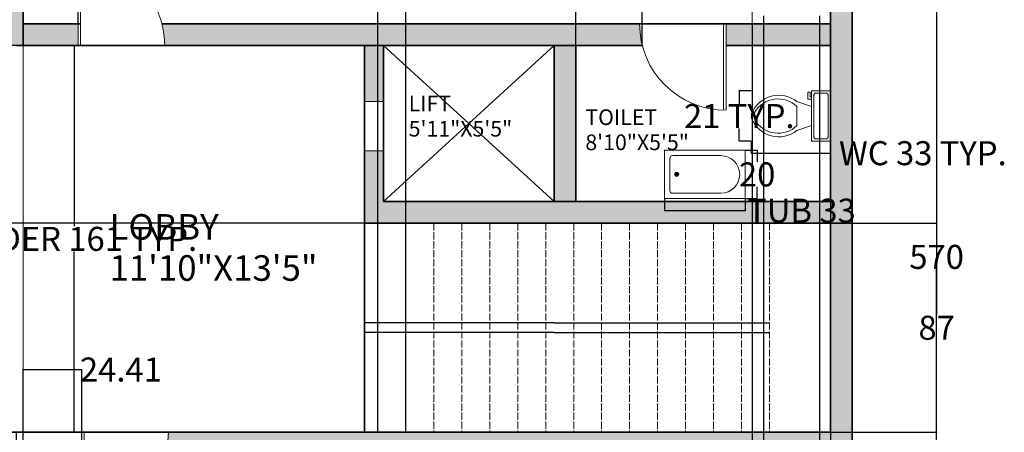
# Model space of a CAD drawing. Units: inches. Extents: x 409 to 1056, y 160 to 945.
# Tile 3 of 6: x 625 to 1035, y 453 to 624. Entities that reach past the tile are written whole.
import ezdxf

# ---------------------------------------------------------------- set-up
doc = ezdxf.new("R2010")
doc.units = ezdxf.units.IN
doc.header["$MEASUREMENT"] = 0
doc.linetypes.add('ACAD_ISO02W100', pattern=[15, 12, -3])
for name, color, linetype, lineweight in [('A-ANNO-DIMS', 2, 'Continuous', 18), ('A-AREA-IDEN', 7, 'Continuous', 18), ('A-DOOR', 3, 'Continuous', 18), ('A-ELEV', 8, 'Continuous', 18), ('A-FLOR-CASE', 8, 'Continuous', 20), ('A-FLOR-FIXT', 8, 'Continuous', 18), ('A-FLOR-STRS', 7, 'Continuous', 25), ('A-FLOR-STRS-TRED', 8, 'ACAD_ISO02W100', 18), ('A-GLAZ', 4, 'Continuous', 18), ('A-WALL', 7, 'Continuous', 35)]:
    doc.layers.add(name, color=color, linetype=linetype, lineweight=lineweight)
doc.layers.add('A-WALL-PATT', color=251, linetype='Continuous', lineweight=13, true_color=0x636466)
doc.styles.get("Standard").update_dxf_attribs({"font": 'arial.ttf'})
doc.dimstyles.get("Standard").update_dxf_attribs({"dimtxt": 10, "dimasz": 0.18, "dimexe": 0.18, "dimexo": 0.0625, "dimgap": 0.09, "dimtad": 0, "dimtih": 1, "dimtoh": 1, "dimdec": 0, "dimzin": 0, "dimdsep": 46, "dimlunit": 3, "dimtxsty": 'Standard', "dimcen": 0.09, "dimadec": 0, "dimazin": 0, "dimtfac": 1, "dimtdec": 0, "dimtofl": 0, "dimtmove": 0, "dimatfit": 3, "dimfxl": 1, "dimtolj": 1, "dimtzin": 0, "dimarcsym": 0})

# ---------------------------------------------------------------- blocks, each defined once
blk = doc.blocks.new('Toilet - top')
for p, q in [((9.5, -6), (9.5, -2)), ((-8, -8.5), (-8, -8)), ((-7, -8), (-7, -9.5)), ((-4, -8), (-6, -14)), ((4, -8), (6, -14)), ((-10, -8.5), (-8, -8.5)), ((-10, -9.5), (-10, -8.5)), ((-7, -9.5), (-10, -9.5)), ((4, -14), (-4, -14))]:
    blk.add_line(p, q)
blk.add_lwpolyline([(10.5, -8), (10.5, 0), (-10.5, 0), (-10.5, -8)], close=True)
for points in [[(-9.5, -2), (-9.5, -6)], [(8.5, -1), (-8.5, -1)], [(-8.5, -7), (8.5, -7)]]:
    blk.add_lwpolyline(points)
for centre, radius, start, end in [((-8.62, -1.88), 0.884, 81.8699, 188.1301), ((8.62, -1.88), 0.884, 351.8699, 98.1301), ((-8.62, -6.12), 0.884, 171.8699, 278.1301), ((8.62, -6.12), 0.884, 261.8699, 8.1301), ((3.52, -21.58), 12.17, 141.4691, 247.9714), ((4.2, -21.82), 11.33, 136.3677, 238.9468), ((-3.52, -21.58), 12.17, 292.0284, 38.5307), ((-4.2, -21.82), 11.33, 301.053, 43.6321), ((0, -27.88), 4, 245.7318, 294.2682), ((0, -29), 4, 254.8605, 285.1395)]:
    blk.add_arc(centre, radius, start, end)
blk = doc.blocks.new('Bath Tub - 26 x 60 in.')
for p, q in [((8, -18), (10, -18)), ((9, -17), (9, -19))]:
    blk.add_line(p, q)
blk.add_lwpolyline([(0, -36), (0, 0), (60, 0), (60, -36)], close=True)
for points in [[(4, -30), (4, -6)], [(6, -4), (42, -4)], [(42, -32), (6, -32)]]:
    blk.add_lwpolyline(points)
for radius in [1.5, 1]:
    blk.add_circle((9, -18), radius)
for centre, radius, start, end in [((5.75, -5.75), 1.77, 81.8699, 188.1301), ((42, -18), 14, 270, 90), ((5.75, -30.25), 1.77, 171.8699, 278.1301)]:
    blk.add_arc(centre, radius, start, end)
blk = doc.blocks.new('DOOR-SWING-36IN')
for p, q in [((35, 36), (35, 0)), ((36, 36), (36, 0))]:
    blk.add_line(p, q)
blk.add_arc((36, 36), 36, 180, 270)
blk = doc.blocks.new('*D13')
at = {"layer": 'A-ANNO-DIMS', "color": 0, "lineweight": -2, "transparency": 16777216}
for p, q in [((623.91, 613.74), (648.18, 613.74)), ((648, 613.56), (648, 538.5)), ((648, 452.92), (648, 527.98)), ((623.91, 452.74), (648.18, 452.74))]:
    blk.add_line(p, q, dxfattribs=at)
at = {"layer": 'A-ANNO-DIMS', "color": 0, "transparency": 16777216}
for points in [[(647.97, 613.56), (648.03, 613.56), (648, 613.74)], [(647.97, 452.92), (648.03, 452.92), (648, 452.74)]]:
    blk.add_solid(points, dxfattribs=at)
at = {"layer": 'Defpoints', "color": 0, "transparency": 16777216}
for p in [(623.85, 613.74), (648, 613.74), (623.85, 452.74)]:
    blk.add_point(p, dxfattribs=at)
at = {"layer": 'A-ANNO-DIMS', "color": 0, "transparency": 16777216, "insert": (648, 533.24), "char_height": 10, "attachment_point": 5}
blk.add_mtext('\\A1;SLIDER 161 TYP.', dxfattribs=at)
blk = doc.blocks.new('*D14')
at = {"layer": 'A-ANNO-DIMS', "color": 0, "lineweight": -2, "transparency": 16777216}
for p, q in [((620.85, 452.68), (620.85, 428.41)), ((623.85, 452.68), (623.85, 428.41)), ((621.03, 428.59), (623.67, 428.59)), ((623.85, 428.59), (624.03, 428.59))]:
    blk.add_line(p, q, dxfattribs=at)
at = {"layer": 'A-ANNO-DIMS', "color": 0, "transparency": 16777216}
for points in [[(621.03, 428.62), (621.03, 428.56), (620.85, 428.59)], [(623.67, 428.62), (623.67, 428.56), (623.85, 428.59)]]:
    blk.add_solid(points, dxfattribs=at)
at = {"layer": 'Defpoints', "color": 0, "transparency": 16777216}
for p in [(620.85, 452.74), (623.85, 452.74), (623.85, 428.59)]:
    blk.add_point(p, dxfattribs=at)
at = {"layer": 'A-ANNO-DIMS', "color": 0, "transparency": 16777216, "insert": (644.57, 428.59), "char_height": 10, "attachment_point": 5}
blk.add_mtext('\\A1;3 TYP.', dxfattribs=at)
blk = doc.blocks.new('*D25')
at = {"layer": 'A-ANNO-DIMS', "color": 0, "lineweight": -2, "transparency": 16777216}
for p, q in [((929.7, 573.78), (929.7, 568.71)), ((962.74, 573.78), (962.74, 568.71)), ((929.88, 568.89), (962.56, 568.89)), ((962.74, 568.89), (962.92, 568.89))]:
    blk.add_line(p, q, dxfattribs=at)
at = {"layer": 'A-ANNO-DIMS', "color": 0, "transparency": 16777216}
for points in [[(929.88, 568.92), (929.88, 568.86), (929.7, 568.89)], [(962.56, 568.92), (962.56, 568.86), (962.74, 568.89)]]:
    blk.add_solid(points, dxfattribs=at)
at = {"layer": 'Defpoints', "color": 0, "transparency": 16777216}
for p in [(929.7, 573.85), (962.74, 573.85), (962.74, 568.89)]:
    blk.add_point(p, dxfattribs=at)
at = {"layer": 'A-ANNO-DIMS', "color": 0, "transparency": 16777216, "insert": (1001.13, 568.89), "char_height": 10, "attachment_point": 5}
blk.add_mtext('\\A1;WC 33 TYP.', dxfattribs=at)
blk = doc.blocks.new('*D26')
at = {"layer": 'A-ANNO-DIMS', "color": 0, "lineweight": -2, "transparency": 16777216}
for p, q in [((929.63, 594.85), (924.56, 594.85)), ((924.74, 594.67), (924.74, 589.46)), ((924.74, 574.03), (924.74, 579.23)), ((929.63, 573.85), (924.56, 573.85))]:
    blk.add_line(p, q, dxfattribs=at)
at = {"layer": 'A-ANNO-DIMS', "color": 0, "transparency": 16777216}
for points in [[(924.71, 594.67), (924.77, 594.67), (924.74, 594.85)], [(924.71, 574.03), (924.77, 574.03), (924.74, 573.85)]]:
    blk.add_solid(points, dxfattribs=at)
at = {"layer": 'Defpoints', "color": 0, "transparency": 16777216}
for p in [(929.7, 594.85), (924.74, 573.85), (929.7, 573.85)]:
    blk.add_point(p, dxfattribs=at)
at = {"layer": 'A-ANNO-DIMS', "color": 0, "transparency": 16777216, "insert": (924.74, 584.35), "char_height": 10, "attachment_point": 5}
blk.add_mtext('\\A1;21 TYP.', dxfattribs=at)
blk = doc.blocks.new('*D27')
at = {"layer": 'A-ANNO-DIMS', "color": 0, "lineweight": -2, "transparency": 16777216}
for p, q in [((893.67, 549.95), (893.67, 544.81)), ((927.15, 549.95), (927.15, 544.81)), ((893.85, 544.99), (926.97, 544.99)), ((927.15, 544.99), (927.33, 544.99))]:
    blk.add_line(p, q, dxfattribs=at)
at = {"layer": 'A-ANNO-DIMS', "color": 0, "transparency": 16777216}
for points in [[(893.85, 545.02), (893.85, 544.96), (893.67, 544.99)], [(926.97, 545.02), (926.97, 544.96), (927.15, 544.99)]]:
    blk.add_solid(points, dxfattribs=at)
at = {"layer": 'Defpoints', "color": 0, "transparency": 16777216}
for p in [(893.67, 550.01), (927.15, 550.01), (927.15, 544.99)]:
    blk.add_point(p, dxfattribs=at)
at = {"layer": 'A-ANNO-DIMS', "color": 0, "transparency": 16777216, "insert": (950.62, 544.99), "char_height": 10, "attachment_point": 5}
blk.add_mtext('\\A1;TUB 33', dxfattribs=at)
blk = doc.blocks.new('*D28')
at = {"layer": 'A-ANNO-DIMS', "color": 0, "lineweight": -2, "transparency": 16777216}
for p, q in [((927.21, 570.1), (932.35, 570.1)), ((932.17, 569.92), (932.17, 565.25)), ((932.17, 550.19), (932.17, 554.86)), ((927.21, 550.01), (932.35, 550.01))]:
    blk.add_line(p, q, dxfattribs=at)
at = {"layer": 'A-ANNO-DIMS', "color": 0, "transparency": 16777216}
for points in [[(932.14, 569.92), (932.2, 569.92), (932.17, 570.1)], [(932.14, 550.19), (932.2, 550.19), (932.17, 550.01)]]:
    blk.add_solid(points, dxfattribs=at)
at = {"layer": 'Defpoints', "color": 0, "transparency": 16777216}
for p in [(927.15, 570.1), (932.17, 570.1), (927.15, 550.01)]:
    blk.add_point(p, dxfattribs=at)
at = {"layer": 'A-ANNO-DIMS', "color": 0, "transparency": 16777216, "insert": (932.17, 560.05), "char_height": 10, "attachment_point": 5}
blk.add_mtext('\\A1;20', dxfattribs=at)
blk = doc.blocks.new('*D38')
at = {"layer": 'A-ANNO-DIMS', "color": 0, "lineweight": -2, "transparency": 16777216}
for p, q in [((971.8, 810.74), (1007.05, 810.74)), ((1006.87, 810.56), (1006.87, 530.94)), ((1006.87, 240.92), (1006.87, 520.55)), ((971.8, 240.74), (1007.05, 240.74))]:
    blk.add_line(p, q, dxfattribs=at)
at = {"layer": 'A-ANNO-DIMS', "color": 0, "transparency": 16777216}
for points in [[(1006.84, 810.56), (1006.9, 810.56), (1006.87, 810.74)], [(1006.84, 240.92), (1006.9, 240.92), (1006.87, 240.74)]]:
    blk.add_solid(points, dxfattribs=at)
at = {"layer": 'Defpoints', "color": 0, "transparency": 16777216}
for p in [(971.74, 810.74), (1006.87, 810.74), (971.74, 240.74)]:
    blk.add_point(p, dxfattribs=at)
at = {"layer": 'A-ANNO-DIMS', "color": 0, "transparency": 16777216, "insert": (1006.87, 525.74), "char_height": 10, "attachment_point": 5}
blk.add_mtext('\\A1;570', dxfattribs=at)
blk = doc.blocks.new('*D40')
at = {"layer": 'A-ANNO-DIMS', "color": 0, "lineweight": -2, "transparency": 16777216}
for p, q in [((930.07, 622.68), (930.07, 166.44)), ((962.74, 622.68), (962.74, 166.44)), ((930.25, 166.62), (962.56, 166.62)), ((962.74, 166.62), (962.92, 166.62))]:
    blk.add_line(p, q, dxfattribs=at)
at = {"layer": 'A-ANNO-DIMS', "color": 0, "transparency": 16777216}
for points in [[(930.25, 166.65), (930.25, 166.59), (930.07, 166.62)], [(962.56, 166.65), (962.56, 166.59), (962.74, 166.62)]]:
    blk.add_solid(points, dxfattribs=at)
at = {"layer": 'Defpoints', "color": 0, "transparency": 16777216}
for p in [(930.07, 622.74), (962.74, 622.74), (962.74, 166.62)]:
    blk.add_point(p, dxfattribs=at)
at = {"layer": 'A-ANNO-DIMS', "color": 0, "transparency": 16777216, "insert": (983.8, 166.62), "char_height": 10, "attachment_point": 5}
blk.add_mtext('\\A1;32.675', dxfattribs=at)
blk = doc.blocks.new('*D41')
at = {"layer": 'A-ANNO-DIMS', "color": 0, "lineweight": -2, "transparency": 16777216}
for p, q in [((934.87, 626.08), (934.87, 166.44)), ((958.09, 626.08), (958.09, 166.44)), ((935.05, 166.62), (957.91, 166.62)), ((958.09, 166.62), (958.27, 166.62))]:
    blk.add_line(p, q, dxfattribs=at)
at = {"layer": 'A-ANNO-DIMS', "color": 0, "transparency": 16777216}
for points in [[(935.05, 166.65), (935.05, 166.59), (934.87, 166.62)], [(957.91, 166.65), (957.91, 166.59), (958.09, 166.62)]]:
    blk.add_solid(points, dxfattribs=at)
at = {"layer": 'Defpoints', "color": 0, "transparency": 16777216}
for p in [(934.87, 626.14), (958.09, 626.14), (958.09, 166.62)]:
    blk.add_point(p, dxfattribs=at)
at = {"layer": 'A-ANNO-DIMS', "color": 0, "transparency": 16777216, "insert": (975.27, 166.62), "char_height": 10, "attachment_point": 5}
blk.add_mtext('\\A1;23.22', dxfattribs=at)
blk = doc.blocks.new('*D49')
at = {"layer": 'A-ANNO-DIMS', "color": 0, "lineweight": -2, "transparency": 16777216}
for p, q in [((937.4, 539.74), (1007.05, 539.74)), ((1006.87, 539.56), (1006.87, 501.44)), ((1006.87, 452.92), (1006.87, 491.05)), ((937.4, 452.74), (1007.05, 452.74))]:
    blk.add_line(p, q, dxfattribs=at)
at = {"layer": 'A-ANNO-DIMS', "color": 0, "transparency": 16777216}
for points in [[(1006.84, 539.56), (1006.9, 539.56), (1006.87, 539.74)], [(1006.84, 452.92), (1006.9, 452.92), (1006.87, 452.74)]]:
    blk.add_solid(points, dxfattribs=at)
at = {"layer": 'Defpoints', "color": 0, "transparency": 16777216}
for p in [(937.34, 539.74), (1006.87, 539.74), (937.34, 452.74)]:
    blk.add_point(p, dxfattribs=at)
at = {"layer": 'A-ANNO-DIMS', "color": 0, "transparency": 16777216, "insert": (1006.87, 496.24), "char_height": 10, "attachment_point": 5}
blk.add_mtext('\\A1;87', dxfattribs=at)
blk = doc.blocks.new('*D51')
at = {"layer": 'A-ANNO-DIMS', "color": 0, "lineweight": -2, "transparency": 16777216}
for p, q in [((856.74, 613.81), (856.74, 939.05)), ((856.92, 938.87), (884.2, 938.87)), ((884.38, 613.81), (884.38, 939.05)), ((884.38, 938.87), (884.56, 938.87))]:
    blk.add_line(p, q, dxfattribs=at)
at = {"layer": 'A-ANNO-DIMS', "color": 0, "transparency": 16777216}
for points in [[(856.92, 938.9), (856.92, 938.84), (856.74, 938.87)], [(884.2, 938.9), (884.2, 938.84), (884.38, 938.87)]]:
    blk.add_solid(points, dxfattribs=at)
at = {"layer": 'Defpoints', "color": 0, "transparency": 16777216}
for p in [(884.38, 938.87), (856.74, 613.74), (884.38, 613.74)]:
    blk.add_point(p, dxfattribs=at)
at = {"layer": 'A-ANNO-DIMS', "color": 0, "transparency": 16777216, "insert": (905.5, 938.87), "char_height": 10, "attachment_point": 5}
blk.add_mtext('\\A1;27.643', dxfattribs=at)
blk = doc.blocks.new('*D52')
at = {"layer": 'A-ANNO-DIMS', "color": 0, "lineweight": -2, "transparency": 16777216}
for p, q in [((768.679251, 613.743876), (420.436751, 613.743876)), ((420.616751, 613.563876), (420.616751, 581.833876)), ((420.616751, 539.923876), (420.616751, 571.653876)), ((768.679251, 539.743876), (420.436751, 539.743876))]:
    blk.add_line(p, q, dxfattribs=at)
at = {"layer": 'A-ANNO-DIMS', "color": 0, "transparency": 16777216}
for points in [[(420.586751, 613.563876), (420.646751, 613.563876), (420.616751, 613.743876)], [(420.586751, 539.923876), (420.646751, 539.923876), (420.616751, 539.743876)]]:
    blk.add_solid(points, dxfattribs=at)
at = {"layer": 'Defpoints', "color": 0, "transparency": 16777216}
for p in [(420.616751, 613.743876), (768.741751, 613.743876), (768.741751, 539.743876)]:
    blk.add_point(p, dxfattribs=at)
at = {"layer": 'A-ANNO-DIMS', "color": 0, "transparency": 16777216, "insert": (420.616751, 576.743876), "char_height": 10, "attachment_point": 5}
blk.add_mtext('\\A1;74', dxfattribs=at)
blk = doc.blocks.new('*D53')
at = {"layer": 'A-ANNO-DIMS', "color": 0, "lineweight": -2, "transparency": 16777216}
for p, q in [((774.31, 452.81), (774.31, 939.05)), ((774.49, 938.87), (785.78, 938.87)), ((785.96, 452.81), (785.96, 939.05)), ((785.96, 938.87), (786.14, 938.87))]:
    blk.add_line(p, q, dxfattribs=at)
at = {"layer": 'A-ANNO-DIMS', "color": 0, "transparency": 16777216}
for points in [[(774.49, 938.9), (774.49, 938.84), (774.31, 938.87)], [(785.78, 938.9), (785.78, 938.84), (785.96, 938.87)]]:
    blk.add_solid(points, dxfattribs=at)
at = {"layer": 'Defpoints', "color": 0, "transparency": 16777216}
for p in [(785.96, 938.87), (774.31, 452.74), (785.96, 452.74)]:
    blk.add_point(p, dxfattribs=at)
at = {"layer": 'A-ANNO-DIMS', "color": 0, "transparency": 16777216, "insert": (806.55, 938.87), "char_height": 10, "attachment_point": 5}
blk.add_mtext('\\A1;11.645', dxfattribs=at)
blk = doc.blocks.new('*D54')
at = {"layer": 'A-ANNO-DIMS', "color": 0, "lineweight": -2, "transparency": 16777216}
for p, q in [((626.74, 622.81), (626.74, 658.05)), ((626.92, 657.87), (649.46, 657.87)), ((649.64, 622.81), (649.64, 658.05)), ((649.64, 657.87), (649.82, 657.87))]:
    blk.add_line(p, q, dxfattribs=at)
at = {"layer": 'A-ANNO-DIMS', "color": 0, "transparency": 16777216}
for points in [[(626.92, 657.9), (626.92, 657.84), (626.74, 657.87)], [(649.46, 657.9), (649.46, 657.84), (649.64, 657.87)]]:
    blk.add_solid(points, dxfattribs=at)
at = {"layer": 'Defpoints', "color": 0, "transparency": 16777216}
for p in [(649.64, 657.87), (626.74, 622.74), (649.64, 622.74)]:
    blk.add_point(p, dxfattribs=at)
at = {"layer": 'A-ANNO-DIMS', "color": 0, "transparency": 16777216, "insert": (663, 657.87), "char_height": 10, "attachment_point": 5}
blk.add_mtext('\\A1;22.9', dxfattribs=at)
blk = doc.blocks.new('*D55')
at = {"layer": 'A-ANNO-DIMS', "color": 0, "lineweight": -2, "transparency": 16777216}
for p, q in [((626.74, 443.81), (626.74, 479.05)), ((626.92, 478.87), (650.97, 478.87)), ((651.15, 443.81), (651.15, 479.05)), ((651.15, 478.87), (651.33, 478.87))]:
    blk.add_line(p, q, dxfattribs=at)
at = {"layer": 'A-ANNO-DIMS', "color": 0, "transparency": 16777216}
for points in [[(626.92, 478.9), (626.92, 478.84), (626.74, 478.87)], [(650.97, 478.9), (650.97, 478.84), (651.15, 478.87)]]:
    blk.add_solid(points, dxfattribs=at)
at = {"layer": 'Defpoints', "color": 0, "transparency": 16777216}
for p in [(651.15, 478.87), (626.74, 443.74), (651.15, 443.74)]:
    blk.add_point(p, dxfattribs=at)
at = {"layer": 'A-ANNO-DIMS', "color": 0, "transparency": 16777216, "insert": (667.41, 478.87), "char_height": 10, "attachment_point": 5}
blk.add_mtext('\\A1;24.41', dxfattribs=at)

msp = doc.modelspace()

# ---------------------------------------------------------------- hatches: boundary and pattern name
at = {"layer": 'A-WALL-PATT'}
h = msp.add_hatch(color=256, dxfattribs=at)
h.dxf.hatch_style = 1
h.paths.add_polyline_path([(626.7418, 801.7439), (870.7418, 801.7439), (870.7418, 710.7439), (870.7418, 683.9043), (875.7418, 683.9043), (875.7418, 707.7439), (962.7418, 707.7439), (962.7418, 710.7439), (875.7418, 710.7439), (875.7418, 722.7439), (875.7418, 801.7439), (885.6955, 801.7439, -0.06325422), (884.5523, 810.7439), (617.7418, 810.7439), (617.7418, 732.9297), (626.7418, 732.9297)])
h.paths.add_polyline_path([(962.7418, 810.7439), (920.5523, 810.7439), (920.5523, 801.7439), (962.7418, 801.7439)], flags=17)
h.paths.add_polyline_path([(971.7418, 810.7439), (962.7418, 810.7439), (962.7418, 801.7439), (962.7418, 707.7439), (962.7418, 622.7439), (962.7418, 613.7439), (962.7418, 548.7439), (856.7418, 548.7439), (847.7418, 548.7439), (776.7418, 548.7439), (776.7418, 569.8172), (768.7418, 569.8172), (768.7418, 539.7439), (847.7418, 539.7439), (971.7418, 539.7439), (971.7418, 613.7439), (971.7418, 707.7439)])
h.paths.add_polyline_path([(883.2418, 622.7439), (875.7418, 622.7439), (684.4993, 622.7439, -0.06325422), (685.6424, 613.7439), (870.7418, 613.7439), (875.7418, 613.7439), (884.3849, 613.7439, -0.06325422)])
h.paths.add_polyline_path([(649.6424, 622.7439), (626.7418, 622.7439), (626.7418, 613.7439), (649.6424, 613.7439)])
h.paths.add_polyline_path([(626.7418, 652.3165), (617.7418, 652.3165), (617.7418, 613.7439), (626.7418, 613.7439), (626.7418, 622.7439)])
h.paths.add_polyline_path([(776.7418, 613.7439), (768.7418, 613.7439), (768.7418, 590.4138), (776.7418, 590.4138)], flags=17)
h.paths.add_polyline_path([(856.7418, 613.7439), (847.7418, 613.7439), (847.7418, 548.7439), (856.7418, 548.7439)], flags=17)
h.paths.add_polyline_path([(962.7418, 622.7439), (919.2418, 622.7439), (919.2418, 613.7439), (962.7418, 613.7439)], flags=17)
h.paths.add_polyline_path([(971.7418, 539.7439), (962.7418, 539.7439), (962.7418, 452.7439), (687.1506, 452.7439, -0.06325422), (686.0074, 443.7439), (962.7418, 443.7439), (962.7418, 331.7439), (927.6873, 331.7439, -0.02784244), (927.9102, 327.7439), (962.7418, 327.7439), (962.7418, 249.7439), (871.7418, 249.7439), (870.7418, 249.7439), (626.7418, 249.7439), (626.7418, 282.7439), (617.7418, 282.7439), (617.7418, 240.7439), (870.7418, 240.7439), (871.7418, 240.7439), (971.7418, 240.7439), (971.7418, 249.7439), (971.7418, 327.7439), (971.7418, 331.7439), (971.7418, 443.7439), (971.7418, 452.7439)])
h.paths.add_polyline_path([(875.7418, 443.7439), (870.7418, 443.7439), (870.7418, 327.7439), (871.7418, 327.7439), (891.9102, 327.7439), (891.9102, 331.7439), (875.7418, 331.7439)], flags=17)

# ---------------------------------------------------------------- linework, layer by layer
at = {"layer": 'A-DOOR'}
for p, q in [((649.6424, 622.7439), (649.6424, 613.7439)), ((919.2418, 622.7439), (883.2418, 622.7439)), ((919.2418, 613.7439), (919.2418, 622.7439)), ((649.6424, 613.7439), (685.6424, 613.7439)), ((651.1506, 452.7439), (651.1506, 443.7439))]:
    msp.add_line(p, q, dxfattribs=at)
at = {"layer": 'A-ELEV'}
for p, q in [((776.7418, 548.7439), (847.7418, 613.7439)), ((847.7418, 548.7439), (776.7418, 613.7439)), ((768.7418, 590.4138), (776.7418, 590.4138)), ((768.7418, 569.8172), (776.7418, 569.8172))]:
    msp.add_line(p, q, dxfattribs=at)
at = {"layer": 'A-FLOR-CASE'}
msp.add_line((930.0665, 707.7439), (930.0665, 622.7439), dxfattribs=at)
at = {"layer": 'A-FLOR-STRS'}
for p, q in [((847.7418, 498.2439), (768.7418, 498.2439)), ((847.7418, 498.2439), (937.1268, 498.2439)), ((847.7418, 494.2439), (768.7418, 494.2439)), ((847.7418, 494.2439), (937.1268, 494.2439))]:
    msp.add_line(p, q, dxfattribs=at)
at = {"layer": 'A-FLOR-STRS-TRED', "ltscale": 0.25}
for p, q in [((774.3113, 539.7439), (774.3113, 452.7439)), ((785.956, 539.7439), (785.956, 452.7439)), ((797.6007, 539.7439), (797.6007, 452.7439)), ((809.2453, 539.7439), (809.2453, 452.7439)), ((820.89, 539.7439), (820.89, 452.7439)), ((832.5347, 539.7439), (832.5347, 452.7439)), ((844.1794, 539.7439), (844.1794, 452.7439)), ((855.8241, 539.7439), (855.8241, 452.7439)), ((867.4688, 539.7439), (867.4688, 452.7439)), ((879.1134, 539.7439), (879.1134, 452.7439)), ((890.7581, 539.7439), (890.7581, 452.7439)), ((902.4028, 539.7439), (902.4028, 452.7439)), ((914.0475, 539.7439), (914.0475, 452.7439)), ((925.6922, 539.7439), (925.6922, 452.7439)), ((937.3368, 539.7439), (937.3368, 452.7439))]:
    msp.add_line(p, q, dxfattribs=at)
at = {"layer": 'A-GLAZ'}
for q in [(617.7418, 613.7439), (626.7418, 452.7439)]:
    msp.add_line((626.7418, 613.7439), q, dxfattribs=at)
at = {"layer": 'A-WALL'}
for p, q in [((626.7418, 801.7439), (626.7418, 622.7439)), ((962.7418, 707.7439), (962.7418, 622.7439)), ((971.7418, 707.7439), (971.7418, 613.7439)), ((626.7418, 622.7439), (650.6424, 622.7439)), ((626.7418, 622.7439), (626.7418, 613.7439)), ((684.4993, 622.7439), (962.7418, 622.7439)), ((962.7418, 622.7439), (875.7418, 622.7439)), ((962.7418, 622.7439), (962.7418, 613.7439)), ((626.7418, 613.7439), (870.7418, 613.7439)), ((768.7418, 452.7439), (768.7418, 613.7439)), ((776.7418, 548.7439), (776.7418, 613.7439)), ((847.7418, 548.7439), (847.7418, 613.7439)), ((856.7418, 548.7439), (856.7418, 613.7439)), ((875.7418, 613.7439), (870.7418, 613.7439)), ((884.3849, 613.7439), (875.7418, 613.7439)), ((962.7418, 613.7439), (919.2418, 613.7439)), ((962.7418, 613.7439), (962.7418, 548.7439)), ((971.7418, 613.7439), (971.7418, 539.7439)), ((847.7418, 548.7439), (776.7418, 548.7439)), ((856.7418, 548.7439), (847.7418, 548.7439)), ((962.7418, 548.7439), (856.7418, 548.7439)), ((847.7418, 539.7439), (768.7418, 539.7439)), ((971.7418, 539.7439), (847.7418, 539.7439)), ((962.7418, 452.7439), (962.7418, 539.7439)), ((971.7418, 452.7439), (971.7418, 539.7439)), ((617.7418, 452.7439), (962.7418, 452.7439)), ((971.7418, 443.7439), (971.7418, 452.7439))]:
    msp.add_line(p, q, dxfattribs=at)

# ---------------------------------------------------------------- block references
at = {"layer": 'A-DOOR', "rotation": 180}
msp.add_blockref('DOOR-SWING-36IN', (685.6428, 649.7438), dxfattribs=at)
at = {"layer": 'A-DOOR'}
msp.add_blockref('DOOR-SWING-36IN', (883.2414, 586.744), dxfattribs=at)
at = {"layer": 'A-DOOR', "extrusion": (0, 0, -1), "zscale": -1}
msp.add_blockref('DOOR-SWING-36IN', (-687.1509, 416.744), dxfattribs=at)
at = {"layer": 'A-FLOR-FIXT', "rotation": 269.9999999999995}
msp.add_blockref('Toilet - top', (962.7418, 584.3475), dxfattribs=at)
at = {"layer": 'A-FLOR-FIXT', "xscale": 0.5579275172153072, "yscale": 0.5579275172153072, "zscale": 0.5579275172153072}
msp.add_blockref('Bath Tub - 26 x 60 in.', (893.6742, 570.0951), dxfattribs=at)

# ---------------------------------------------------------------- texts
at = {"layer": 'A-AREA-IDEN'}
for s, height, p in [('LIFT', 6.50615, (787.1762, 586.2613)), ('TOILET ', 6.50615, (860.6905, 580.6165)), ('5\'11"X5\'5"', 6.50615, (787.1762, 575.8097)), ('8\'10"X5\'5"', 6.50615, (860.6905, 570.1649)), ('LOBBY', 10.64286, (662.6424, 532.893)), ('11\'10"X13\'5"', 10.642856, (662.6424, 515.7962))]:
    msp.add_text(s, height=height, dxfattribs=at).set_placement(p)

# ---------------------------------------------------------------- dimensions: what is measured, and where the dimension line sits
at = {"layer": 'A-ANNO-DIMS'}
for base, p1, p2, override, picture, middle in [((785.956, 938.8689), (774.3113, 452.7439), (785.956, 452.7439), {"dimdec": 3, "dimlfac": 1, "dimrnd": 0, "dimzin": 0, "dimdsep": 46, "dimlunit": 2}, '*D53', (806.55, 938.8689)), ((884.3849, 938.8689), (856.7418, 613.7439), (884.3849, 613.7439), {"dimdec": 3, "dimlfac": 1, "dimrnd": 0, "dimzin": 0, "dimdsep": 46, "dimlunit": 2}, '*D51', (905.4973, 938.8689)), ((649.6424, 657.8689), (626.7418, 622.7439), (649.6424, 622.7439), {"dimdec": 1, "dimlfac": 1, "dimrnd": 0, "dimzin": 0, "dimdsep": 46, "dimlunit": 2}, '*D54', (662.9956, 657.8689)), ((958.0915, 166.6189), (934.8736, 626.1427), (958.0915, 626.1427), {"dimdec": 2, "dimlfac": 1, "dimrnd": 0, "dimzin": 0, "dimdsep": 46, "dimlunit": 2}, '*D41', (975.2681, 166.6189)), ((962.7418, 166.6189), (930.0665, 622.7439), (962.7418, 622.7439), {"dimdec": 3, "dimlfac": 1, "dimrnd": 0, "dimzin": 0, "dimdsep": 46, "dimlunit": 2}, '*D40', (983.803, 166.6189)), ((651.1506, 478.8689), (626.7418, 443.7439), (651.1506, 443.7439), {"dimdec": 2, "dimlfac": 1, "dimrnd": 0, "dimzin": 0, "dimdsep": 46, "dimlunit": 2}, '*D55', (667.4131, 478.8689))]:
    dim = msp.add_linear_dim(base=base, p1=p1, p2=p2, dimstyle='Standard', override=override, dxfattribs=at)
    dim.commit()
    dim.dimension.update_dxf_attribs({"geometry": picture, "text_midpoint": middle})
for base, p1, p2, picture, middle in [((1006.8668, 810.7439), (971.7418, 240.7439), (971.7418, 810.7439), '*D38', (1006.8668, 525.7439)), ((420.6168, 613.7439), (768.7418, 539.7439), (768.7418, 613.7439), '*D52', (420.6168, 576.7439)), ((932.1712, 570.0951), (927.1499, 550.0097), (927.1499, 570.0951), '*D28', (932.1712, 560.0524)), ((1006.8668, 539.7439), (937.3368, 452.7439), (937.3368, 539.7439), '*D49', (1006.8668, 496.2439))]:
    dim = msp.add_linear_dim(base=base, p1=p1, p2=p2, angle=90, dimstyle='Standard', override={"dimdec": 0, "dimlfac": 1, "dimrnd": 0, "dimzin": 0, "dimdsep": 46, "dimlunit": 2}, dxfattribs=at)
    dim.commit()
    dim.dimension.update_dxf_attribs({"geometry": picture, "text_midpoint": middle})
for base, p1, p2, angle, text, picture, middle in [((647.9987, 613.7439), (623.8487, 452.7439), (623.8487, 613.7439), 90, 'SLIDER <> TYP.', '*D13', (647.9987, 533.2439)), ((924.7386, 573.8475), (929.6955, 594.8475), (929.6955, 573.8475), 270, '<> TYP.', '*D26', (924.7386, 584.3475))]:
    dim = msp.add_linear_dim(base=base, p1=p1, p2=p2, angle=angle, text=text, dimstyle='Standard', override={"dimdec": 0, "dimlfac": 1, "dimrnd": 0, "dimzin": 0, "dimdsep": 46, "dimlunit": 2}, dxfattribs=at)
    dim.commit()
    dim.dimension.update_dxf_attribs({"geometry": picture, "text_midpoint": middle})
for base, p1, p2, text, picture, middle in [((962.7418, 568.8905), (929.6955, 573.8475), (962.7418, 573.8475), 'WC <> TYP.', '*D25', (1001.1325, 568.8905)), ((927.1499, 544.9884), (893.6742, 550.0097), (927.1499, 550.0097), 'TUB <>', '*D27', (950.619, 544.9884)), ((623.8487, 428.5939), (620.8487, 452.7439), (623.8487, 452.7439), '<> TYP.', '*D14', (644.5689, 428.5939))]:
    dim = msp.add_linear_dim(base=base, p1=p1, p2=p2, text=text, dimstyle='Standard', override={"dimdec": 0, "dimlfac": 1, "dimrnd": 0, "dimzin": 0, "dimdsep": 46, "dimlunit": 2}, dxfattribs=at)
    dim.commit()
    dim.dimension.update_dxf_attribs({"geometry": picture, "text_midpoint": middle})

doc.saveas('drawing.dxf')
